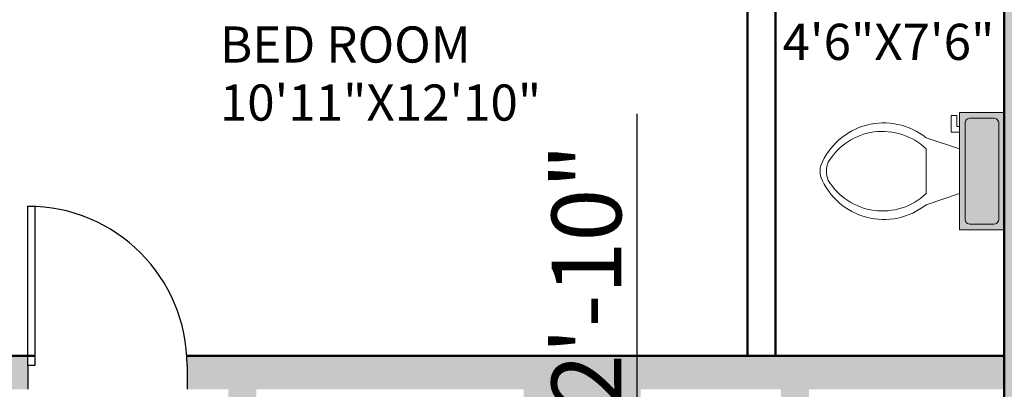
# Model space of a CAD drawing. Units: inches. Extents: x 2419 to 2878, y 1068 to 1713.
# Tile 16 of 20: x 2595 to 2772, y 1409 to 1475. Entities that reach past the tile are written whole.
import ezdxf

# ---------------------------------------------------------------- set-up
doc = ezdxf.new("R2010")
doc.units = ezdxf.units.IN
for name, color, linetype, lineweight in [('A-ANNO-DIMS', 2, 'Continuous', 18), ('A-AREA-IDEN', 7, 'Continuous', 18), ('A-DOOR', 4, 'Continuous', 25), ('A-FLOR-FIXT', 8, 'Continuous', 18), ('A-FLOR-PRKG-PATT', 1, 'Continuous', 13), ('A-FURN-PATT', 254, 'Continuous', 13), ('A-WALL', 7, 'Continuous', 50)]:
    doc.layers.add(name, color=color, linetype=linetype, lineweight=lineweight)
doc.layers.add('A-FLOR-FIXT-PATT', color=254, linetype='Continuous', lineweight=13, true_color=0xd7ebd2)
doc.layers.add('A-WALL-PATT', color=18, linetype='Continuous', lineweight=13, true_color=0x000000)
doc.styles.get("Standard").update_dxf_attribs({"font": 'arial.ttf'})
doc.dimstyles.new('ISO-25', dxfattribs={"dimtxt": 12.5, "dimasz": 2.5, "dimexe": 1.25, "dimexo": 0.625, "dimtad": 1, "dimdec": 0, "dimlunit": 4, "dimtxsty": 'Standard', "dimblk": 'ARCHTICK', "dimcen": 2.5, "dimse1": 1, "dimse2": 1, "dimclrd": 4, "dimadec": 0, "dimazin": 0, "dimtfac": 1, "dimtdec": 0, "dimtmove": 0, "dimatfit": 3, "dimfxl": 1, "dimarcsym": 0})

# ---------------------------------------------------------------- blocks, each defined once
blk = doc.blocks.new('*U5')
for p, q in [((9.5, -6), (9.5, -2)), ((-10, -8.5), (-8, -8.5)), ((-10, -9.5), (-10, -8.5)), ((-8, -8.5), (-8, -8)), ((-7, -8), (-7, -9.5)), ((-4, -8), (-6, -14)), ((4, -8), (6, -14)), ((-7, -9.5), (-10, -9.5)), ((4, -14), (-4, -14))]:
    blk.add_line(p, q)
blk.add_lwpolyline([(10.5, -8), (10.5, 0), (-10.5, 0), (-10.5, -8)], close=True)
for points in [[(8.5, -1), (-8.5, -1)], [(-9.5, -2), (-9.5, -6)], [(-8.5, -7), (8.5, -7)]]:
    blk.add_lwpolyline(points)
for centre, radius, start, end in [((-8.62, -1.88), 0.884, 81.8699, 188.1301), ((8.62, -1.88), 0.884, 351.8699, 98.1301), ((-8.62, -6.12), 0.884, 171.8699, 278.1301), ((8.62, -6.12), 0.884, 261.8699, 8.1301), ((3.52, -21.58), 12.17, 141.4691, 247.9714), ((4.2, -21.82), 11.33, 136.3677, 238.9468), ((-3.52, -21.58), 12.17, 292.0284, 38.5307), ((-4.2, -21.82), 11.33, 301.053, 43.6321), ((0, -27.88), 4, 245.7318, 294.2682), ((0, -29), 4, 254.8605, 285.1395)]:
    blk.add_arc(centre, radius, start, end)
blk = doc.blocks.new('*U3')
for p, q in [((0, 0), (0, -6)), ((40, 0), (40, -6))]:
    blk.add_line(p, q)
blk.add_lwpolyline([(0, 0), (0, 40), (1.75, 40), (1.75, 0)], close=True)
blk.add_arc((0, 0), 40, 0, 90)
blk = doc.blocks.new('_ArchTick')
at = {"color": 0, "linetype": 'ByBlock', "const_width": 0.15}
blk.add_lwpolyline([(-0.5, -0.5), (0.5, 0.5)], dxfattribs=at)
blk = doc.blocks.new('*D21')
at = {"layer": 'A-ANNO-DIMS', "color": 4, "lineweight": -2, "transparency": 16777216}
for p, q in [((2624.02, 1390.72), (2632.51, 1390.72)), ((2632.51, 1390.72), (2741.59, 1390.72))]:
    blk.add_line(p, q, dxfattribs=at)
at = {"layer": 'Defpoints', "color": 0, "transparency": 16777216}
for p in [(2624.02, 1392.52), (2632.51, 1392.52), (2632.51, 1390.72)]:
    blk.add_point(p, dxfattribs=at)
at = {"layer": 'A-ANNO-DIMS', "color": 4, "lineweight": -2, "transparency": 16777216, "xscale": 2.5, "yscale": 2.5, "zscale": 2.5, "rotation": 180}
blk.add_blockref('_ArchTick', (2624.02, 1390.72), dxfattribs=at)
at = {"layer": 'A-ANNO-DIMS', "color": 4, "lineweight": -2, "transparency": 16777216, "xscale": 2.5, "yscale": 2.5, "zscale": 2.5}
blk.add_blockref('_ArchTick', (2632.51, 1390.72), dxfattribs=at)
at = {"layer": 'A-ANNO-DIMS', "color": 0, "transparency": 16777216, "insert": (2688.3, 1397.81), "char_height": 12.5, "attachment_point": 5}
blk.add_mtext('0\'-8 1/2" TYP.', dxfattribs=at)
blk = doc.blocks.new('*D32')
at = {"layer": 'A-ANNO-DIMS', "color": 4, "lineweight": -2, "transparency": 16777216}
for p, q in [((2705.74, 1272.77), (2705.74, 1458.17)), ((2705.74, 1238.68), (2705.74, 1272.77))]:
    blk.add_line(p, q, dxfattribs=at)
at = {"layer": 'Defpoints', "color": 0, "transparency": 16777216}
for p in [(2705.74, 1272.77), (2710.85, 1272.77), (2710.85, 1238.68)]:
    blk.add_point(p, dxfattribs=at)
at = {"layer": 'A-ANNO-DIMS', "color": 4, "lineweight": -2, "transparency": 16777216, "xscale": 2.5, "yscale": 2.5, "zscale": 2.5}
for p, rotation in [((2705.74, 1272.77), 90), ((2705.74, 1238.68), 270)]:
    blk.add_blockref('_ArchTick', p, dxfattribs=dict(at, rotation=rotation))
at = {"layer": 'A-ANNO-DIMS', "color": 0, "transparency": 16777216, "insert": (2698.27, 1366.72), "char_height": 12.5, "attachment_point": 5, "rotation": 90}
blk.add_mtext('SQUARE TABLE 2\'-10"', dxfattribs=at)
blk = doc.blocks.new('*D36')
at = {"layer": 'A-ANNO-DIMS', "color": 4, "lineweight": -2, "transparency": 16777216}
blk.add_line((2656.74, 1605.01), (2736.32, 1605.01), dxfattribs=at)
at = {"layer": 'Defpoints', "color": 0, "transparency": 16777216}
for p in [(2736.32, 1605.01), (2656.74, 1205.81), (2736.32, 1205.81)]:
    blk.add_point(p, dxfattribs=at)
at = {"layer": 'A-ANNO-DIMS', "color": 4, "lineweight": -2, "transparency": 16777216, "xscale": 2.5, "yscale": 2.5, "zscale": 2.5, "rotation": 180}
blk.add_blockref('_ArchTick', (2656.74, 1605.01), dxfattribs=at)
at = {"layer": 'A-ANNO-DIMS', "color": 4, "lineweight": -2, "transparency": 16777216, "xscale": 2.5, "yscale": 2.5, "zscale": 2.5}
blk.add_blockref('_ArchTick', (2736.32, 1605.01), dxfattribs=at)
at = {"layer": 'A-ANNO-DIMS', "color": 0, "transparency": 16777216, "insert": (2696.53, 1612.1), "char_height": 12.5, "attachment_point": 5}
blk.add_mtext('6\'-7 1/2"', dxfattribs=at)
blk = doc.blocks.new('*D37')
at = {"layer": 'A-ANNO-DIMS', "color": 4, "lineweight": -2, "transparency": 16777216}
for p, q in [((2736.32, 1605.01), (2771.51, 1605.01)), ((2771.51, 1605.01), (2818.42, 1605.01))]:
    blk.add_line(p, q, dxfattribs=at)
at = {"layer": 'Defpoints', "color": 0, "transparency": 16777216}
for p in [(2771.51, 1605.01), (2736.32, 1205.81), (2771.51, 1205.81)]:
    blk.add_point(p, dxfattribs=at)
at = {"layer": 'A-ANNO-DIMS', "color": 4, "lineweight": -2, "transparency": 16777216, "xscale": 2.5, "yscale": 2.5, "zscale": 2.5, "rotation": 180}
blk.add_blockref('_ArchTick', (2736.32, 1605.01), dxfattribs=at)
at = {"layer": 'A-ANNO-DIMS', "color": 4, "lineweight": -2, "transparency": 16777216, "xscale": 2.5, "yscale": 2.5, "zscale": 2.5}
blk.add_blockref('_ArchTick', (2771.51, 1605.01), dxfattribs=at)
at = {"layer": 'A-ANNO-DIMS', "color": 0, "transparency": 16777216, "insert": (2796.22, 1611.91), "char_height": 12.5, "attachment_point": 5}
blk.add_mtext('2\'-11"', dxfattribs=at)
blk = doc.blocks.new('*D39')
at = {"layer": 'A-ANNO-DIMS', "color": 4, "lineweight": -2, "transparency": 16777216}
for p, q in [((2662.74, 1605.01), (2668.59, 1605.01)), ((2668.59, 1605.01), (2705.56, 1605.01))]:
    blk.add_line(p, q, dxfattribs=at)
at = {"layer": 'Defpoints', "color": 0, "transparency": 16777216}
for p in [(2668.59, 1605.01), (2662.74, 1165.6), (2668.59, 1165.6)]:
    blk.add_point(p, dxfattribs=at)
at = {"layer": 'A-ANNO-DIMS', "color": 4, "lineweight": -2, "transparency": 16777216, "xscale": 2.5, "yscale": 2.5, "zscale": 2.5, "rotation": 180}
blk.add_blockref('_ArchTick', (2662.74, 1605.01), dxfattribs=at)
at = {"layer": 'A-ANNO-DIMS', "color": 4, "lineweight": -2, "transparency": 16777216, "xscale": 2.5, "yscale": 2.5, "zscale": 2.5}
blk.add_blockref('_ArchTick', (2668.59, 1605.01), dxfattribs=at)
at = {"layer": 'A-ANNO-DIMS', "color": 0, "transparency": 16777216, "insert": (2688.32, 1612.02), "char_height": 12.5, "attachment_point": 5}
blk.add_mtext('0\'-6"', dxfattribs=at)
blk = doc.blocks.new('*D50')
at = {"layer": 'A-ANNO-DIMS', "color": 4, "lineweight": -2, "transparency": 16777216}
for p, q in [((2444.31, 1458.39), (2444.31, 1494.19)), ((2444.31, 1437.39), (2444.31, 1458.39))]:
    blk.add_line(p, q, dxfattribs=at)
at = {"layer": 'Defpoints', "color": 0, "transparency": 16777216}
for p in [(2444.31, 1458.39), (2763.51, 1458.39), (2763.51, 1437.39)]:
    blk.add_point(p, dxfattribs=at)
at = {"layer": 'A-ANNO-DIMS', "color": 4, "lineweight": -2, "transparency": 16777216, "xscale": 2.5, "yscale": 2.5, "zscale": 2.5}
for p, rotation in [((2444.31, 1458.39), 90), ((2444.31, 1437.39), 270)]:
    blk.add_blockref('_ArchTick', p, dxfattribs=dict(at, rotation=rotation))
at = {"layer": 'A-ANNO-DIMS', "color": 0, "transparency": 16777216, "insert": (2437.31, 1477.54), "char_height": 12.5, "attachment_point": 5, "rotation": 90}
blk.add_mtext('1\'-9"', dxfattribs=at)
blk = doc.blocks.new('*D51')
at = {"layer": 'A-ANNO-DIMS', "color": 4, "lineweight": -2, "transparency": 16777216}
for p, q in [((2738.51, 1079.92), (2771.51, 1079.92)), ((2771.51, 1079.92), (2808.71, 1079.92))]:
    blk.add_line(p, q, dxfattribs=at)
at = {"layer": 'Defpoints', "color": 0, "transparency": 16777216}
for p in [(2738.51, 1447.89), (2771.51, 1437.39), (2771.51, 1079.92)]:
    blk.add_point(p, dxfattribs=at)
at = {"layer": 'A-ANNO-DIMS', "color": 4, "lineweight": -2, "transparency": 16777216, "xscale": 2.5, "yscale": 2.5, "zscale": 2.5, "rotation": 180}
blk.add_blockref('_ArchTick', (2738.51, 1079.92), dxfattribs=at)
at = {"layer": 'A-ANNO-DIMS', "color": 4, "lineweight": -2, "transparency": 16777216, "xscale": 2.5, "yscale": 2.5, "zscale": 2.5}
blk.add_blockref('_ArchTick', (2771.51, 1079.92), dxfattribs=at)
at = {"layer": 'A-ANNO-DIMS', "color": 0, "transparency": 16777216, "insert": (2791.36, 1086.93), "char_height": 12.5, "attachment_point": 5}
blk.add_mtext('2\'-9"', dxfattribs=at)
blk = doc.blocks.new('*D53')
at = {"layer": 'A-ANNO-DIMS', "color": 4, "lineweight": -2, "transparency": 16777216}
for p, q in [((2638.79, 1605.01), (2667.31, 1605.01)), ((2667.31, 1605.01), (2733.63, 1605.01))]:
    blk.add_line(p, q, dxfattribs=at)
at = {"layer": 'Defpoints', "color": 0, "transparency": 16777216}
for p in [(2667.31, 1605.01), (2638.79, 1217.38), (2667.31, 1217.38)]:
    blk.add_point(p, dxfattribs=at)
at = {"layer": 'A-ANNO-DIMS', "color": 4, "lineweight": -2, "transparency": 16777216, "xscale": 2.5, "yscale": 2.5, "zscale": 2.5, "rotation": 180}
blk.add_blockref('_ArchTick', (2638.79, 1605.01), dxfattribs=at)
at = {"layer": 'A-ANNO-DIMS', "color": 4, "lineweight": -2, "transparency": 16777216, "xscale": 2.5, "yscale": 2.5, "zscale": 2.5}
blk.add_blockref('_ArchTick', (2667.31, 1605.01), dxfattribs=at)
at = {"layer": 'A-ANNO-DIMS', "color": 0, "transparency": 16777216, "insert": (2701.72, 1612.1), "char_height": 12.5, "attachment_point": 5}
blk.add_mtext('2\'-4 1/2"', dxfattribs=at)
blk = doc.blocks.new('*D61')
at = {"layer": 'A-ANNO-DIMS', "color": 4, "lineweight": -2, "transparency": 16777216}
blk.add_line((2730.51, 1079.92), (2771.51, 1079.92), dxfattribs=at)
at = {"layer": 'Defpoints', "color": 0, "transparency": 16777216}
for p in [(2730.51, 1414.81), (2771.51, 1414.81), (2771.51, 1079.92)]:
    blk.add_point(p, dxfattribs=at)
at = {"layer": 'A-ANNO-DIMS', "color": 4, "lineweight": -2, "transparency": 16777216, "xscale": 2.5, "yscale": 2.5, "zscale": 2.5, "rotation": 180}
blk.add_blockref('_ArchTick', (2730.51, 1079.92), dxfattribs=at)
at = {"layer": 'A-ANNO-DIMS', "color": 4, "lineweight": -2, "transparency": 16777216, "xscale": 2.5, "yscale": 2.5, "zscale": 2.5}
blk.add_blockref('_ArchTick', (2771.51, 1079.92), dxfattribs=at)
at = {"layer": 'A-ANNO-DIMS', "color": 0, "transparency": 16777216, "insert": (2751.01, 1086.94), "char_height": 12.5, "attachment_point": 5}
blk.add_mtext('3\'-5"', dxfattribs=at)

msp = doc.modelspace()

# ---------------------------------------------------------------- hatches: boundary and pattern name
at = {"layer": 'A-FLOR-FIXT-PATT'}
h = msp.add_hatch(color=256, dxfattribs=at)
h.dxf.hatch_style = 1
h.paths.add_polyline_path([(2705.38, 1406.81, 0.5), (2704.38, 1407.81), (2687.38, 1407.81, 0.5), (2686.38, 1406.81), (2686.38, 1402.81, 0.5), (2687.38, 1401.81), (2704.38, 1401.81, 0.5), (2705.38, 1402.81)])
h.paths.add_polyline_path([(2770.51, 1456.39, 0.5), (2769.51, 1457.39), (2765.51, 1457.39, 0.5), (2764.51, 1456.39), (2764.51, 1439.39, 0.5), (2765.51, 1438.39), (2769.51, 1438.39, 0.5), (2770.51, 1439.39)])
h.paths.add_polyline_path([(2641.68, 1567.61), (2662.48, 1567.61), (2662.48, 1554.41), (2664.88, 1554.41), (2664.88, 1567.61), (2685.68, 1567.61), (2685.68, 1552.41), (2680.48, 1552.41), (2693.68, 1539.21), (2693.68, 1568.81), (2633.68, 1568.81), (2633.68, 1554.41), (2641.68, 1554.41)])
h.paths.add_polyline_path([(2678.48, 1554.41), (2678.48, 1539.21), (2693.68, 1539.21)], flags=17)
h = msp.add_hatch(color=256, dxfattribs=at)
h.dxf.hatch_style = 1
h.paths.add_polyline_path([(2771.51, 1458.39), (2763.51, 1458.39), (2763.51, 1437.39), (2771.51, 1437.39)])
h.paths.add_polyline_path([(2770.51, 1456.39, 0.5), (2769.51, 1457.39), (2765.51, 1457.39, 0.5), (2764.51, 1456.39), (2764.51, 1439.39, 0.5), (2765.51, 1438.39), (2769.51, 1438.39, 0.5), (2770.51, 1439.39)], flags=16)
h.paths.add_polyline_path([(2706.38, 1408.81), (2685.38, 1408.81), (2685.38, 1400.81), (2706.38, 1400.81)])
h.paths.add_polyline_path([(2704.38, 1401.81, 0.5), (2705.38, 1402.81), (2705.38, 1406.81, 0.5), (2704.38, 1407.81), (2687.38, 1407.81, 0.5), (2686.38, 1406.81), (2686.38, 1402.81, 0.5), (2687.38, 1401.81)], flags=16)
h.paths.add_polyline_path([(2574.48, 1207.45), (2633.94, 1207.45), (2633.94, 1217.37), (2574.48, 1217.37)], flags=9)
h.paths.add_polyline_path([(2574.45, 1217.83), (2610.47, 1217.83), (2610.47, 1227.88), (2574.45, 1227.88)], flags=9)
h.paths.add_polyline_path([(2672.43, 1304.02), (2718.62, 1304.02), (2718.62, 1313.94), (2672.43, 1313.94)], flags=9)
h.paths.add_polyline_path([(2672.4, 1314.4), (2750.13, 1314.4), (2750.13, 1324.45), (2672.4, 1324.45)], flags=9)
h.paths.add_polyline_path([(2500.43, 1374.44), (2544.8, 1374.44), (2544.8, 1384.36), (2500.43, 1384.36)], flags=9)
h.paths.add_polyline_path([(2500.41, 1384.82), (2566.08, 1384.82), (2566.08, 1394.87), (2500.41, 1394.87)], flags=9)
h.paths.add_polyline_path([(2738.93, 1376.75), (2778.27, 1376.75), (2778.27, 1386.67), (2738.93, 1386.67)], flags=9)
h.paths.add_polyline_path([(2659.12, 1357.8), (2703.49, 1357.8), (2703.49, 1367.72), (2659.12, 1367.72)], flags=9)
h.paths.add_polyline_path([(2659.1, 1368.18), (2694.11, 1368.18), (2694.11, 1378.23), (2659.1, 1378.23)], flags=9)
h.paths.add_polyline_path([(2730.12, 1466.07), (2769.46, 1466.07), (2769.46, 1475.99), (2730.12, 1475.99)], flags=9)
h.paths.add_polyline_path([(2730.1, 1476.45), (2765.12, 1476.45), (2765.12, 1486.5), (2730.1, 1486.5)], flags=9)
h.paths.add_polyline_path([(2730.38, 1518.65), (2761.48, 1518.65), (2761.48, 1528.57), (2730.38, 1528.57)], flags=9)
h.paths.add_polyline_path([(2730.36, 1529.03), (2780.96, 1529.03), (2780.96, 1539.07), (2730.36, 1539.07)], flags=9)
h.paths.add_polyline_path([(2629.32, 1455.19), (2688.78, 1455.19), (2688.78, 1465.11), (2629.32, 1465.11)], flags=9)
h.paths.add_polyline_path([(2629.3, 1465.57), (2681.9, 1465.57), (2681.9, 1475.62), (2629.3, 1475.62)], flags=9)
h.paths.add_polyline_path([(2513.23, 1456.48), (2562.63, 1456.48), (2562.63, 1466.4), (2513.23, 1466.4)], flags=9)
h.paths.add_polyline_path([(2513.21, 1466.86), (2556.26, 1466.86), (2556.26, 1476.91), (2513.21, 1476.91)], flags=9)
h.paths.add_polyline_path([(2488.87, 1521.54), (2519.97, 1521.54), (2519.97, 1531.46), (2488.87, 1531.46)], flags=9)
h.paths.add_polyline_path([(2536.55, 1543.51), (2580.92, 1543.51), (2580.92, 1553.43), (2536.55, 1553.43)], flags=9)
h.paths.add_polyline_path([(2536.56, 1553.92), (2573.53, 1553.92), (2573.53, 1563.8), (2536.56, 1563.8)], flags=9)
at = {"layer": 'A-FLOR-PRKG-PATT'}
h = msp.add_hatch(color=256, dxfattribs=at)
h.dxf.hatch_style = 1
edge = h.paths.add_edge_path()
edge.add_ellipse((2561.37, 1279.45), major_axis=(3.99, 0), ratio=0.842304, start_angle=0.6466, end_angle=90)
edge.add_line((2561.37, 1282.81), (2511.57, 1282.81))
edge.add_ellipse((2511.57, 1279.45), major_axis=(3.99, 0), ratio=0.842304, start_angle=90, end_angle=179.3534)
edge.add_ellipse((10560.89, 1188.62), major_axis=(-8054.03, 0), ratio=0.8423039, start_angle=-0.646554, end_angle=-0.628237)
edge.add_ellipse((2509.23, 1276.91), major_axis=(1.69, 0), ratio=0.842304, start_angle=179.3718, end_angle=248.4648)
edge.add_ellipse((10560.33, 1188.62), major_axis=(8052.29, 0), ratio=0.8423039, start_angle=179.353446, end_angle=179.381357, ccw=False)
edge.add_ellipse((2511.01, 1279.45), major_axis=(2.25, 0), ratio=0.842304, start_angle=90, end_angle=179.3534, ccw=False)
edge.add_line((2511.01, 1281.35), (2561.94, 1281.35))
edge.add_ellipse((2561.94, 1279.45), major_axis=(-2.25, 0), ratio=0.842304, start_angle=180.6466, end_angle=270, ccw=False)
edge.add_ellipse((-5487.38, 1188.62), major_axis=(8052.29, 0), ratio=0.8423039, start_angle=0.528271, end_angle=0.646554, ccw=False)
edge.add_ellipse((2563.71, 1276.91), major_axis=(-1.69, 0), ratio=0.842304, start_angle=111.5352, end_angle=180.6282)
edge.add_ellipse((-5487.95, 1188.62), major_axis=(-8054.03, 0), ratio=0.8423039, start_angle=180.628237, end_angle=180.646554)
edge = h.paths.add_edge_path()
edge.add_ellipse((2564.91, 1261.91), major_axis=(-1.12, 0), ratio=0.842304, start_angle=180, end_angle=270)
edge.add_line((2564.91, 1262.86), (2564.43, 1262.86))
edge.add_ellipse((-5487.38, 1188.62), major_axis=(8052.29, 0), ratio=0.8423039, start_angle=0.383867, end_angle=0.528271, ccw=False)
edge.add_line((2564.65, 1242.56), (2564.91, 1242.56))
edge.add_ellipse((2564.91, 1243.51), major_axis=(-1.12, 0), ratio=0.842304, start_angle=90, end_angle=180)
edge.add_line((2566.03, 1243.51), (2566.03, 1261.91))
edge = h.paths.add_edge_path()
edge.add_ellipse((2564.91, 1174.99), major_axis=(1.12, 0), ratio=0.842304, start_angle=0, end_angle=90)
edge.add_line((2564.91, 1175.94), (2564.89, 1175.94))
edge.add_ellipse((-5487.38, 1188.62), major_axis=(8052.29, 0), ratio=0.8423039, start_angle=-0.134987, end_angle=-0.090229, ccw=False)
edge.add_ellipse((2163.34, 1170.91), major_axis=(401.54, 0), ratio=0.842304, start_angle=-2.18, end_angle=-0.1356, ccw=False)
edge.add_line((2564.47, 1155.64), (2564.91, 1155.64))
edge.add_ellipse((2564.91, 1156.59), major_axis=(-1.12, 0), ratio=0.842304, start_angle=90, end_angle=180)
edge.add_line((2566.03, 1156.59), (2566.03, 1174.99))
h.paths.add_polyline_path([(2574.48, 1207.45), (2633.94, 1207.45), (2633.94, 1217.37), (2574.48, 1217.37)], flags=9)
h.paths.add_polyline_path([(2574.45, 1217.83), (2610.47, 1217.83), (2610.47, 1227.88), (2574.45, 1227.88)], flags=9)
h.paths.add_polyline_path([(2672.43, 1304.02), (2718.62, 1304.02), (2718.62, 1313.94), (2672.43, 1313.94)], flags=9)
h.paths.add_polyline_path([(2672.4, 1314.4), (2750.13, 1314.4), (2750.13, 1324.45), (2672.4, 1324.45)], flags=9)
h.paths.add_polyline_path([(2500.43, 1374.44), (2544.8, 1374.44), (2544.8, 1384.36), (2500.43, 1384.36)], flags=9)
h.paths.add_polyline_path([(2500.41, 1384.82), (2566.08, 1384.82), (2566.08, 1394.87), (2500.41, 1394.87)], flags=9)
h.paths.add_polyline_path([(2738.93, 1376.75), (2778.27, 1376.75), (2778.27, 1386.67), (2738.93, 1386.67)], flags=9)
h.paths.add_polyline_path([(2659.12, 1357.8), (2703.49, 1357.8), (2703.49, 1367.72), (2659.12, 1367.72)], flags=9)
h.paths.add_polyline_path([(2659.1, 1368.18), (2694.11, 1368.18), (2694.11, 1378.23), (2659.1, 1378.23)], flags=9)
h.paths.add_polyline_path([(2730.12, 1466.07), (2769.46, 1466.07), (2769.46, 1475.99), (2730.12, 1475.99)], flags=9)
h.paths.add_polyline_path([(2730.1, 1476.45), (2765.12, 1476.45), (2765.12, 1486.5), (2730.1, 1486.5)], flags=9)
h.paths.add_polyline_path([(2730.38, 1518.65), (2761.48, 1518.65), (2761.48, 1528.57), (2730.38, 1528.57)], flags=9)
h.paths.add_polyline_path([(2730.36, 1529.03), (2780.96, 1529.03), (2780.96, 1539.07), (2730.36, 1539.07)], flags=9)
h.paths.add_polyline_path([(2629.32, 1455.19), (2688.78, 1455.19), (2688.78, 1465.11), (2629.32, 1465.11)], flags=9)
h.paths.add_polyline_path([(2629.3, 1465.57), (2681.9, 1465.57), (2681.9, 1475.62), (2629.3, 1475.62)], flags=9)
h.paths.add_polyline_path([(2513.23, 1456.48), (2562.63, 1456.48), (2562.63, 1466.4), (2513.23, 1466.4)], flags=9)
h.paths.add_polyline_path([(2513.21, 1466.86), (2556.26, 1466.86), (2556.26, 1476.91), (2513.21, 1476.91)], flags=9)
h.paths.add_polyline_path([(2488.87, 1521.54), (2519.97, 1521.54), (2519.97, 1531.46), (2488.87, 1531.46)], flags=9)
h.paths.add_polyline_path([(2536.55, 1543.51), (2580.92, 1543.51), (2580.92, 1553.43), (2536.55, 1553.43)], flags=9)
h.paths.add_polyline_path([(2536.56, 1553.92), (2573.53, 1553.92), (2573.53, 1563.8), (2536.56, 1563.8)], flags=9)
at = {"layer": 'A-FURN-PATT'}
h = msp.add_hatch(color=256, dxfattribs=at)
h.dxf.hatch_style = 1
h.paths.add_polyline_path([(2710.17, 1562.64), (2707.17, 1559.64), (2709.17, 1559.64, -0.414214), (2710.17, 1560.64)])
h.paths.add_polyline_path([(2711.17, 1559.64, 1), (2709.17, 1559.64, 1)])
h.paths.add_polyline_path([(2710.17, 1562.64), (2710.17, 1560.64, -0.414214), (2711.17, 1559.64), (2713.17, 1559.64)])
h.paths.add_polyline_path([(2713.17, 1559.64), (2711.17, 1559.64, -0.414214), (2710.17, 1558.64), (2710.17, 1556.64)])
h.paths.add_polyline_path([(2710.17, 1558.64, -0.414214), (2709.17, 1559.64), (2707.17, 1559.64), (2710.17, 1556.64)])
h.paths.add_polyline_path([(2613.13, 1558.89, 1), (2611.13, 1558.89, 1)])
h.paths.add_polyline_path([(2612.13, 1561.89), (2612.13, 1559.89, -0.414214), (2613.13, 1558.89), (2615.13, 1558.89)])
h.paths.add_polyline_path([(2612.13, 1559.89), (2612.13, 1561.89), (2609.13, 1558.89), (2611.13, 1558.89, -0.414214)])
h.paths.add_polyline_path([(2612.13, 1557.89, -0.414214), (2611.13, 1558.89), (2609.13, 1558.89), (2612.13, 1555.89)])
h.paths.add_polyline_path([(2574.48, 1207.45), (2633.94, 1207.45), (2633.94, 1217.37), (2574.48, 1217.37)], flags=9)
h.paths.add_polyline_path([(2574.45, 1217.83), (2610.47, 1217.83), (2610.47, 1227.88), (2574.45, 1227.88)], flags=9)
h.paths.add_polyline_path([(2672.43, 1304.02), (2718.62, 1304.02), (2718.62, 1313.94), (2672.43, 1313.94)], flags=9)
h.paths.add_polyline_path([(2672.4, 1314.4), (2750.13, 1314.4), (2750.13, 1324.45), (2672.4, 1324.45)], flags=9)
h.paths.add_polyline_path([(2500.43, 1374.44), (2544.8, 1374.44), (2544.8, 1384.36), (2500.43, 1384.36)], flags=9)
h.paths.add_polyline_path([(2500.41, 1384.82), (2566.08, 1384.82), (2566.08, 1394.87), (2500.41, 1394.87)], flags=9)
h.paths.add_polyline_path([(2738.93, 1376.75), (2778.27, 1376.75), (2778.27, 1386.67), (2738.93, 1386.67)], flags=9)
h.paths.add_polyline_path([(2659.12, 1357.8), (2703.49, 1357.8), (2703.49, 1367.72), (2659.12, 1367.72)], flags=9)
h.paths.add_polyline_path([(2659.1, 1368.18), (2694.11, 1368.18), (2694.11, 1378.23), (2659.1, 1378.23)], flags=9)
h.paths.add_polyline_path([(2730.12, 1466.07), (2769.46, 1466.07), (2769.46, 1475.99), (2730.12, 1475.99)], flags=9)
h.paths.add_polyline_path([(2730.1, 1476.45), (2765.12, 1476.45), (2765.12, 1486.5), (2730.1, 1486.5)], flags=9)
h.paths.add_polyline_path([(2730.38, 1518.65), (2761.48, 1518.65), (2761.48, 1528.57), (2730.38, 1528.57)], flags=9)
h.paths.add_polyline_path([(2730.36, 1529.03), (2780.96, 1529.03), (2780.96, 1539.07), (2730.36, 1539.07)], flags=9)
h.paths.add_polyline_path([(2629.32, 1455.19), (2688.78, 1455.19), (2688.78, 1465.11), (2629.32, 1465.11)], flags=9)
h.paths.add_polyline_path([(2629.3, 1465.57), (2681.9, 1465.57), (2681.9, 1475.62), (2629.3, 1475.62)], flags=9)
h.paths.add_polyline_path([(2513.23, 1456.48), (2562.63, 1456.48), (2562.63, 1466.4), (2513.23, 1466.4)], flags=9)
h.paths.add_polyline_path([(2513.21, 1466.86), (2556.26, 1466.86), (2556.26, 1476.91), (2513.21, 1476.91)], flags=9)
h.paths.add_polyline_path([(2488.87, 1521.54), (2519.97, 1521.54), (2519.97, 1531.46), (2488.87, 1531.46)], flags=9)
h.paths.add_polyline_path([(2536.55, 1543.51), (2580.92, 1543.51), (2580.92, 1553.43), (2536.55, 1553.43)], flags=9)
h.paths.add_polyline_path([(2536.56, 1553.92), (2573.53, 1553.92), (2573.53, 1563.8), (2536.56, 1563.8)], flags=9)
at = {"layer": 'A-WALL-PATT'}
h = msp.add_hatch(color=256, dxfattribs=at)
h.dxf.hatch_style = 1
h.paths.add_polyline_path([(2780.51, 1577.81), (2471.51, 1577.81), (2471.51, 1121.81), (2780.51, 1121.81)])
h.paths.add_polyline_path([(2480.51, 1568.81), (2771.51, 1568.81), (2771.51, 1130.81), (2480.51, 1130.81)], flags=16)
h.paths.add_polyline_path([(2528.51, 1568.81), (2528.51, 1512.81), (2594.51, 1512.81), (2594.51, 1414.81), (2596.57, 1414.81), (2596.57, 1441.61), (2597.82, 1441.61), (2597.82, 1441.58, -0.384016), (2625.03, 1414.81), (2725.51, 1414.81), (2725.51, 1567.55), (2728.3, 1567.55), (2746.89, 1567.55), (2746.89, 1566.73), (2746.87, 1566.73, -0.367216), (2730.51, 1549.09), (2730.51, 1512.81), (2750.85, 1512.81), (2750.85, 1510.03, -0.401453), (2733.08, 1491.46), (2733.08, 1491.44), (2732.27, 1491.44), (2732.27, 1507.81), (2730.51, 1507.81), (2730.51, 1408.81), (2736.51, 1408.81), (2736.51, 1349.81), (2632.51, 1349.81), (2632.51, 1408.81), (2528.51, 1408.81), (2528.51, 1414.81), (2503.97, 1414.81), (2503.97, 1494.85), (2558.38, 1494.85), (2558.38, 1507.81), (2529.96, 1507.81, -0.414214), (2530.82, 1506.96), (2530.82, 1497.26, -0.414214), (2529.96, 1496.4), (2514.56, 1496.4, -0.414214), (2513.7, 1497.26), (2513.7, 1506.96, -0.414214), (2514.56, 1507.81), (2528.51, 1507.81), (2528.51, 1512.81), (2480.51, 1512.81)], flags=0)
h.paths.add_polyline_path([(2516.26, 1507.81), (2528.26, 1507.81), (2528.26, 1505.81), (2523.42, 1505.81), (2524.07, 1504.67), (2529.39, 1504.67, -0.414214), (2529.96, 1504.1), (2529.96, 1497.83, -0.414214), (2529.39, 1497.26), (2515.13, 1497.26, -0.414214), (2514.56, 1497.83), (2514.56, 1504.1, -0.414214), (2515.13, 1504.67), (2520.69, 1504.67), (2521.34, 1505.81), (2516.26, 1505.81)], flags=0)
h.paths.add_polyline_path([(2522.02, 1505.53), (2522.82, 1507.32, -0.65506), (2522.25, 1506.06), (2522.19, 1505.93), (2522.43, 1505.53)], flags=0)
h.paths.add_polyline_path([(2522.83, 1500.97, -1), (2521.69, 1500.97, -1)], flags=0)
h.paths.add_polyline_path([(2522.55, 1500.97, -1), (2521.98, 1500.97, -1)], flags=0)
h.paths.add_polyline_path([(2482.01, 1470.63), (2499.89, 1470.63), (2499.89, 1448.27), (2482.01, 1448.27), (2482.01, 1452.74), (2481.26, 1452.74), (2481.26, 1449.76), (2480.51, 1449.76), (2480.51, 1469.14), (2481.26, 1469.14), (2481.26, 1466.16), (2482.01, 1466.16)], flags=0)
h.paths.add_polyline_path([(2488.71, 1466.16, -1), (2484.24, 1466.16, -1)], flags=0)
h.paths.add_polyline_path([(2496.17, 1466.16, -1), (2490.2, 1466.16, -1)], flags=0)
h.paths.add_polyline_path([(2487.97, 1466.16, -1), (2484.99, 1466.16, -1)], flags=0)
h.paths.add_polyline_path([(2495.42, 1466.16, -1), (2490.95, 1466.16, -1)], flags=0)
h.paths.add_polyline_path([(2487.22, 1466.16, -1), (2485.73, 1466.16, -1)], flags=0)
h.paths.add_polyline_path([(2494.68, 1466.16, -1), (2491.69, 1466.16, -1)], flags=0)
h.paths.add_polyline_path([(2499.11, 1468, -1), (2497.98, 1468, -1)], flags=0)
h.paths.add_polyline_path([(2493.93, 1466.16, -1), (2492.44, 1466.16, -1)], flags=0)
h.paths.add_polyline_path([(2499.37, 1463.71, -1), (2498.17, 1463.71, -1)], flags=0)
h.paths.add_polyline_path([(2484.24, 1461.69), (2496.17, 1461.69), (2496.17, 1457.22), (2484.24, 1457.22)], flags=0)
h.paths.add_polyline_path([(2484.99, 1460.94), (2495.42, 1460.94), (2495.42, 1457.96), (2484.99, 1457.96)], flags=0)
h.paths.add_polyline_path([(2586.88, 1510.03), (2587.69, 1510.03), (2587.69, 1491.44), (2586.88, 1491.44)], flags=0)
h.paths.add_polyline_path([(2499.26, 1459.41, -1), (2498.2, 1459.41, -1)], flags=0)
h.paths.add_polyline_path([(2489.46, 1452.74, -1), (2483.5, 1452.74, -1)], flags=0)
h.paths.add_polyline_path([(2557.3, 1408.81), (2557.3, 1413.09, -0.401453), (2584.57, 1441.58), (2584.57, 1441.61), (2585.82, 1441.61), (2585.82, 1413.09), (2585.82, 1408.81)], flags=0)
h.paths.add_polyline_path([(2488.71, 1452.74, -1), (2484.24, 1452.74, -1)], flags=0)
h.paths.add_polyline_path([(2495.42, 1452.74, -1), (2490.95, 1452.74, -1)], flags=0)
h.paths.add_polyline_path([(2487.97, 1452.74, -1), (2484.99, 1452.74, -1)], flags=0)
h.paths.add_polyline_path([(2494.68, 1452.74, -1), (2491.69, 1452.74, -1)], flags=0)
h.paths.add_polyline_path([(2487.22, 1452.74, -1), (2485.73, 1452.74, -1)], flags=0)
h.paths.add_polyline_path([(2499.18, 1454.44, -1), (2497.9, 1454.44, -1)], flags=0)
h.paths.add_polyline_path([(2493.93, 1452.74, -1), (2492.44, 1452.74, -1)], flags=0)
h.paths.add_polyline_path([(2499.3, 1450.64, -1), (2497.79, 1450.64, -1)], flags=0)
h.paths.add_polyline_path([(2619.13, 1558.89, -1), (2605.13, 1558.89, -1)], flags=0)
h.paths.add_polyline_path([(2609.13, 1558.89), (2612.13, 1561.89), (2615.13, 1558.89), (2612.13, 1555.89)], flags=0)
h.paths.add_polyline_path([(2611.13, 1558.89, -1), (2613.13, 1558.89, -1)], flags=0)
h.paths.add_polyline_path([(2633.68, 1568.81), (2693.68, 1568.81), (2693.68, 1488.81), (2633.68, 1488.81)], flags=0)
h.paths.add_polyline_path([(2641.68, 1554.41), (2641.68, 1567.61), (2662.48, 1567.61), (2662.48, 1554.41), (2664.88, 1554.41), (2664.88, 1567.61), (2685.68, 1567.61), (2685.68, 1552.41), (2680.48, 1552.41), (2693.68, 1539.21), (2678.48, 1539.21), (2678.48, 1554.41)], flags=0)
h.paths.add_polyline_path([(2637.51, 1408.81), (2731.51, 1408.81), (2731.51, 1354.81), (2637.51, 1354.81), (2637.51, 1357.98), (2635.3, 1357.98), (2635.3, 1358.79), (2637.51, 1358.79)], flags=0)
h.paths.add_polyline_path([(2717.17, 1559.64, -1), (2703.17, 1559.64, -1)], flags=0)
h.paths.add_polyline_path([(2707.17, 1559.64), (2710.17, 1562.64), (2713.17, 1559.64), (2710.17, 1556.64)], flags=0)
h.paths.add_polyline_path([(2709.17, 1559.64, -1), (2711.17, 1559.64, -1)], flags=0)
h.paths.add_polyline_path([(2685.38, 1408.81), (2706.38, 1408.81), (2706.38, 1400.81), (2699.88, 1400.81), (2701.88, 1394.81, -0.501323), (2696.92, 1375.95, -0.132891), (2694.83, 1375.95, -0.501317), (2689.88, 1394.81), (2691.88, 1400.81), (2688.88, 1400.81), (2688.88, 1399.31), (2685.88, 1399.31), (2685.88, 1400.31), (2687.88, 1400.31), (2687.88, 1400.81), (2685.38, 1400.81)], flags=0)
h.paths.add_polyline_path([(2687.38, 1407.81), (2704.38, 1407.81, -0.5), (2705.38, 1406.81), (2705.38, 1402.81, -0.5), (2704.38, 1401.81), (2687.38, 1401.81, -0.5), (2686.38, 1402.81), (2686.38, 1406.81, -0.5)], flags=0)
h.paths.add_polyline_path([(2639.51, 1205.81), (2634.51, 1205.81), (2634.51, 1293.81), (2637.51, 1293.81), (2639.51, 1293.81)], flags=0)
h.paths.add_polyline_path([(2691.88, 1394.81), (2699.88, 1394.81, -0.48008), (2697.52, 1377.29, -0.215004), (2694.23, 1377.29, -0.48008)], flags=0)
h.paths.add_polyline_path([(2757.51, 1453.89), (2763.51, 1451.89), (2763.51, 1454.89), (2762.01, 1454.89), (2762.01, 1457.89), (2763.01, 1457.89), (2763.01, 1455.89), (2763.51, 1455.89), (2763.51, 1458.39), (2771.51, 1458.39), (2771.51, 1437.39), (2763.51, 1437.39), (2763.51, 1443.89), (2757.51, 1441.89, -0.501323), (2738.65, 1446.85, -0.132891), (2738.65, 1448.94, -0.501317)], flags=0)
h.paths.add_polyline_path([(2739.99, 1449.54, -0.48008), (2757.51, 1451.89), (2757.51, 1443.89, -0.48008), (2739.99, 1446.25, -0.215004)], flags=0)
h.paths.add_polyline_path([(2765.51, 1457.39), (2769.51, 1457.39, -0.5), (2770.51, 1456.39), (2770.51, 1439.39, -0.5), (2769.51, 1438.39), (2765.51, 1438.39, -0.5), (2764.51, 1439.39), (2764.51, 1456.39, -0.5)], flags=0)
h = msp.add_hatch(color=256, dxfattribs=at)
h.dxf.hatch_style = 1
h.paths.add_polyline_path([(2771.51, 1354.81), (2736.51, 1354.81), (2736.51, 1408.81), (2771.51, 1408.81), (2771.51, 1414.81), (2625.03, 1414.81, -0.015108), (2625.09, 1413.09), (2625.09, 1408.81), (2632.51, 1408.81), (2632.51, 1376.56), (2635.3, 1376.56, -0.029838), (2637.51, 1376.43), (2637.51, 1408.81), (2731.51, 1408.81), (2731.51, 1354.81), (2637.51, 1354.81), (2637.51, 1357.98), (2635.3, 1357.98), (2632.51, 1357.98), (2632.51, 1349.81), (2771.51, 1349.81)])
h.paths.add_polyline_path([(2639.51, 1298.81), (2637.51, 1298.81), (2480.51, 1298.81), (2480.51, 1293.81), (2637.51, 1293.81), (2639.51, 1293.81)])
h.paths.add_polyline_path([(2639.51, 1293.81), (2637.51, 1293.81), (2634.51, 1293.81), (2634.51, 1244.65), (2638.79, 1244.65, -0.006332), (2639.51, 1244.64)])
h.paths.add_polyline_path([(2639.51, 1205.81), (2771.51, 1205.81), (2771.51, 1210.81), (2639.51, 1210.81), (2639.51, 1216.13), (2638.79, 1216.13), (2634.51, 1216.13), (2634.51, 1130.81), (2639.51, 1130.81)])
h.paths.add_polyline_path([(2596.57, 1413.09), (2596.57, 1414.81), (2585.82, 1414.81), (2585.82, 1413.09), (2585.82, 1408.81), (2596.57, 1408.81)])
h.paths.add_polyline_path([(2557.3, 1413.09, -0.015108), (2557.35, 1414.81), (2480.51, 1414.81), (2480.51, 1408.81), (2557.3, 1408.81)])
h.paths.add_polyline_path([(2574.48, 1207.45), (2633.94, 1207.45), (2633.94, 1217.37), (2574.48, 1217.37)], flags=9)
h.paths.add_polyline_path([(2574.45, 1217.83), (2610.47, 1217.83), (2610.47, 1227.88), (2574.45, 1227.88)], flags=9)
h.paths.add_polyline_path([(2672.43, 1304.02), (2718.62, 1304.02), (2718.62, 1313.94), (2672.43, 1313.94)], flags=9)
h.paths.add_polyline_path([(2672.4, 1314.4), (2750.13, 1314.4), (2750.13, 1324.45), (2672.4, 1324.45)], flags=9)
h.paths.add_polyline_path([(2500.43, 1374.44), (2544.8, 1374.44), (2544.8, 1384.36), (2500.43, 1384.36)], flags=9)
h.paths.add_polyline_path([(2500.41, 1384.82), (2566.08, 1384.82), (2566.08, 1394.87), (2500.41, 1394.87)], flags=9)
h.paths.add_polyline_path([(2738.93, 1376.75), (2778.27, 1376.75), (2778.27, 1386.67), (2738.93, 1386.67)], flags=9)
h.paths.add_polyline_path([(2659.12, 1357.8), (2703.49, 1357.8), (2703.49, 1367.72), (2659.12, 1367.72)], flags=25)
h.paths.add_polyline_path([(2659.1, 1368.18), (2694.11, 1368.18), (2694.11, 1378.23), (2659.1, 1378.23)], flags=25)
h.paths.add_polyline_path([(2730.12, 1466.07), (2769.46, 1466.07), (2769.46, 1475.99), (2730.12, 1475.99)], flags=9)
h.paths.add_polyline_path([(2730.1, 1476.45), (2765.12, 1476.45), (2765.12, 1486.5), (2730.1, 1486.5)], flags=9)
h.paths.add_polyline_path([(2730.38, 1518.65), (2761.48, 1518.65), (2761.48, 1528.57), (2730.38, 1528.57)], flags=9)
h.paths.add_polyline_path([(2730.36, 1529.03), (2780.96, 1529.03), (2780.96, 1539.07), (2730.36, 1539.07)], flags=9)
h.paths.add_polyline_path([(2629.32, 1455.19), (2688.78, 1455.19), (2688.78, 1465.11), (2629.32, 1465.11)], flags=9)
h.paths.add_polyline_path([(2629.3, 1465.57), (2681.9, 1465.57), (2681.9, 1475.62), (2629.3, 1475.62)], flags=9)
h.paths.add_polyline_path([(2513.23, 1456.48), (2562.63, 1456.48), (2562.63, 1466.4), (2513.23, 1466.4)], flags=9)
h.paths.add_polyline_path([(2513.21, 1466.86), (2556.26, 1466.86), (2556.26, 1476.91), (2513.21, 1476.91)], flags=9)
h.paths.add_polyline_path([(2488.87, 1521.54), (2519.97, 1521.54), (2519.97, 1531.46), (2488.87, 1531.46)], flags=9)
h.paths.add_polyline_path([(2536.55, 1543.51), (2580.92, 1543.51), (2580.92, 1553.43), (2536.55, 1553.43)], flags=9)
h.paths.add_polyline_path([(2536.56, 1553.92), (2573.53, 1553.92), (2573.53, 1563.8), (2536.56, 1563.8)], flags=9)

# ---------------------------------------------------------------- linework, layer by layer
at = {"layer": 'A-WALL'}
for p, q in [((2771.51, 1568.81), (2771.51, 1130.81)), ((2725.51, 1414.81), (2725.51, 1548.96)), ((2730.51, 1414.81), (2730.51, 1507.81)), ((2584.57, 1414.81), (2597.82, 1414.81)), ((2625.03, 1414.81), (2771.51, 1414.81))]:
    msp.add_line(p, q, dxfattribs=at)

# ---------------------------------------------------------------- block references
at = {"layer": 'A-DOOR', "xscale": 0.712964811120882, "yscale": 0.712964811120882, "zscale": 0.712964811120882}
msp.add_blockref('*U3', (2596.57, 1413.09), dxfattribs=at)
at = {"layer": 'A-FLOR-FIXT', "rotation": 270}
msp.add_blockref('*U5', (2771.51, 1447.89), dxfattribs=at)

# ---------------------------------------------------------------- texts
at = {"layer": 'A-AREA-IDEN'}
for s, height, p in [('BED ROOM', 6.475, (2630.97, 1467.35)), ('4\'6"X7\'6"', 6.475, (2731.78, 1467.83)), ('10\'11"X12\'10"', 6.4753, (2630.97, 1456.95))]:
    msp.add_text(s, height=height, dxfattribs=at).set_placement(p)

# ---------------------------------------------------------------- dimensions: what is measured, and where the dimension line sits
at = {"layer": 'A-ANNO-DIMS'}
for base, p1, p2, picture, middle in [((2667.31, 1605.01), (2638.79, 1217.38), (2667.31, 1217.38), '*D53', (2701.72, 1612.1)), ((2736.32, 1605.01), (2656.74, 1205.81), (2736.32, 1205.81), '*D36', (2696.53, 1612.1)), ((2668.5856, 1605.013), (2662.7408, 1165.6026), (2668.5856, 1165.6026), '*D39', (2688.3247, 1612.0201)), ((2771.51, 1605.01), (2736.32, 1205.81), (2771.51, 1205.81), '*D37', (2796.22, 1611.91)), ((2771.51, 1079.92), (2738.51, 1447.89), (2771.51, 1437.39), '*D51', (2791.36, 1086.93)), ((2771.51, 1079.92), (2730.51, 1414.81), (2771.51, 1414.81), '*D61', (2751.01, 1086.94))]:
    dim = msp.add_linear_dim(base=base, p1=p1, p2=p2, dimstyle='ISO-25', override={"dimdec": 1, "dimlfac": 1, "dimrnd": 0, "dimzin": 1, "dimdsep": 46, "dimlunit": 4, "dimfrac": 2}, dxfattribs=at)
    dim.commit()
    dim.dimension.update_dxf_attribs({"geometry": picture, "text_midpoint": middle})
dim = msp.add_linear_dim(base=(2444.31, 1458.39), p1=(2763.51, 1437.39), p2=(2763.51, 1458.39), angle=90, dimstyle='ISO-25', override={"dimdec": 1, "dimlfac": 1, "dimrnd": 0, "dimzin": 1, "dimdsep": 46, "dimlunit": 4, "dimfrac": 2}, dxfattribs=at)
dim.commit()
dim.dimension.update_dxf_attribs({"geometry": '*D50', "text_midpoint": (2437.31, 1477.54)})
dim = msp.add_linear_dim(base=(2705.74, 1272.77), p1=(2710.85, 1238.68), p2=(2710.85, 1272.77), angle=90, text='SQUARE TABLE <>', dimstyle='ISO-25', override={"dimdec": 1, "dimlfac": 1, "dimrnd": 0, "dimzin": 1, "dimdsep": 46, "dimlunit": 4, "dimfrac": 2}, dxfattribs=at)
dim.commit()
dim.dimension.update_dxf_attribs({"geometry": '*D32', "text_midpoint": (2698.27, 1366.72)})
dim = msp.add_linear_dim(base=(2632.51, 1390.72), p1=(2624.02, 1392.52), p2=(2632.51, 1392.52), text='<> TYP.', dimstyle='ISO-25', override={"dimdec": 1, "dimlfac": 1, "dimrnd": 0, "dimzin": 1, "dimdsep": 46, "dimlunit": 4, "dimfrac": 2}, dxfattribs=at)
dim.commit()
dim.dimension.update_dxf_attribs({"geometry": '*D21', "text_midpoint": (2688.3, 1397.81)})

doc.saveas('drawing.dxf')
